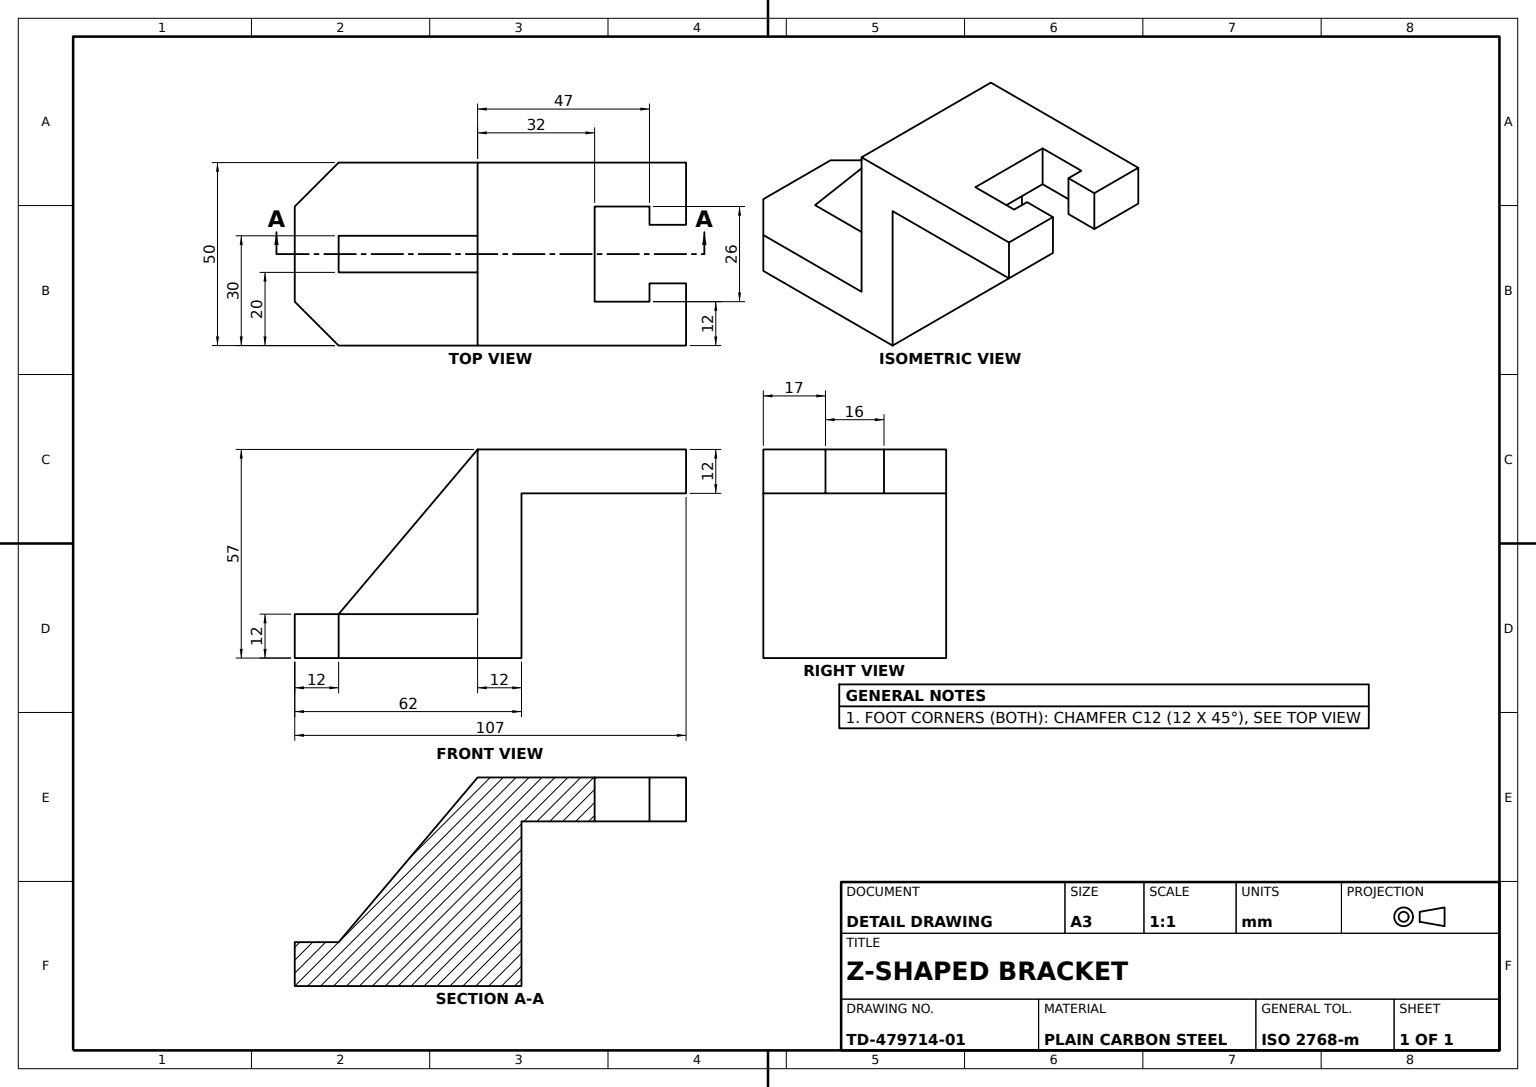
from build123d import *

# Parameters (mm, degrees)
BRACKET_BODY_50MM_DEPTH    = 50
STEP_POCKET_12MM_DEPTH     = 12
SLOT_CUT_12MM_DEPTH        = 12
TRIANGULAR_BOSS_30MM_DEPTH = 30
TRIANGULAR_CUT_20MM_DEPTH  = 20


with BuildPart() as part:
    # Bracket Body Profile → Bracket Body 50mm (new body)
    with BuildSketch(Plane.XY):
        Polygon((0, 0), (12, 0), (62, 0), (62, 45), (107, 45), (107, 57), (50, 57), (50, 12), (12, 12), (0, 12), align=None)
    extrude(amount=BRACKET_BODY_50MM_DEPTH)

    # Step Pocket Profile → Step Pocket 12mm (cut)
    with BuildSketch(Plane(origin=(0, 12, 0), x_dir=(1, 0, 0), z_dir=(0, 1, 0))):
        Polygon((0, -12), (0, 0), (12, 0), align=None)
        Polygon((0, -50), (0, -38), (12, -50), align=None)
    extrude(amount=-STEP_POCKET_12MM_DEPTH, mode=Mode.SUBTRACT)

    # Slot Cut Profile → Slot Cut 12mm (cut)
    with BuildSketch(Plane(origin=(0, 57, 0), x_dir=(1, 0, 0), z_dir=(0, 1, 0))):
        Polygon((107, -25), (107, -17), (97, -17), (97, -12), (82, -12), (82, -38), (97, -38), (97, -33), (107, -33), align=None)
    extrude(amount=-SLOT_CUT_12MM_DEPTH, mode=Mode.SUBTRACT)

    # Triangular Boss Profile → Triangular Boss 30mm (add)
    with BuildSketch(Plane.XY.offset(50)):
        Polygon((12, 12), (50, 12), (50, 57), align=None)
    extrude(amount=-TRIANGULAR_BOSS_30MM_DEPTH)

    # Triangular Cut Profile → Triangular Cut 20mm (cut)
    with BuildSketch(Plane.XY.offset(50)):
        Polygon((12, 12), (50, 57), (50, 12), align=None)
    extrude(amount=-TRIANGULAR_CUT_20MM_DEPTH, mode=Mode.SUBTRACT)


solid = part.part
